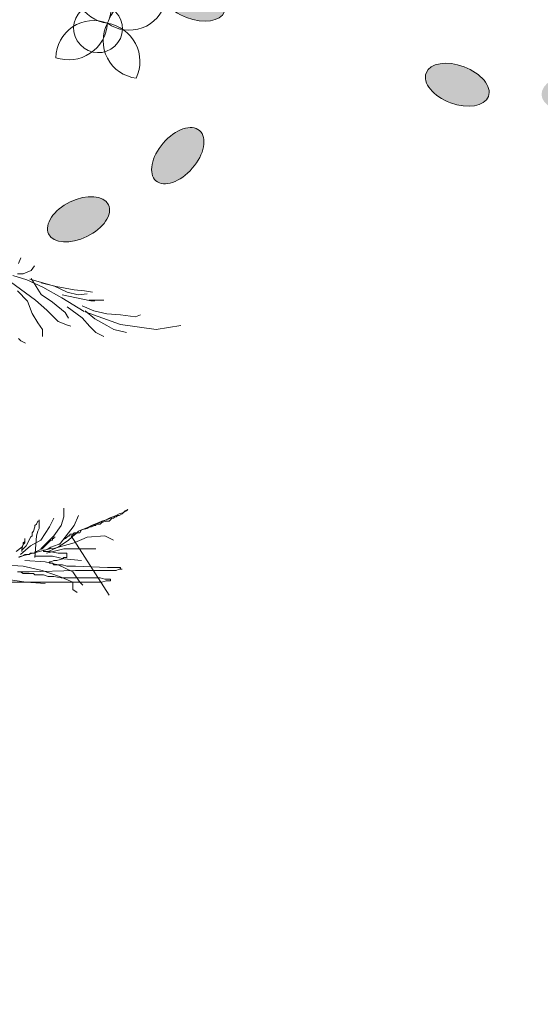
# Model space of a CAD drawing. Units: millimetres. Extents: x 595116 to 630915, y 909473 to 920225.
# Tile 75 of 134: x 629636.47 to 629646.73, y 919266.51 to 919285.9. Entities that reach past the tile are written whole.
import ezdxf

# ---------------------------------------------------------------- set-up
doc = ezdxf.new("R2010")
doc.units = ezdxf.units.MM
doc.layers.add('Dimension', color=3, linetype='Continuous', lineweight=18)
doc.layers.add('L-PLNT', color=85, linetype='Continuous', lineweight=13)
doc.styles.get("Standard").update_dxf_attribs({"font": 'arial.ttf'})
doc.dimstyles.new('ISO-25', dxfattribs={"dimtxt": 9, "dimasz": 6, "dimexe": 1.25, "dimexo": 0.625, "dimtad": 1, "dimlunit": 4, "dimtxsty": 'Standard', "dimcen": 2.5, "dimadec": 0, "dimazin": 0, "dimtfac": 1, "dimtmove": 0, "dimatfit": 3, "dimfxl": 1, "dimarcsym": 0})

# ---------------------------------------------------------------- blocks, each defined once
blk = doc.blocks.new('A$C4FB75ABC')
for p, q in [((4.5963, 3.4774), (4.6082, 3.5072)), ((4.6619, 3.4416), (4.6798, 3.4655)), ((4.5657, 3.4153), (4.6395, 3.3917)), ((4.5903, 3.4238), (4.6201, 3.4238)), ((4.6201, 3.4238), (4.6619, 3.4416)), ((4.5545, 3.382), (4.6858, 3.2866)), ((4.6395, 3.3917), (4.7247, 3.3534)), ((4.6551, 3.396), (4.7847, 3.3597)), ((4.6619, 3.3999), (4.7156, 3.3164)), ((4.7156, 3.3761), (4.7931, 3.3582)), ((4.7847, 3.3597), (4.8521, 3.3286)), ((4.7931, 3.3582), (4.8886, 3.3403)), ((4.5903, 3.3343), (4.644, 3.2807)), ((4.7156, 3.3164), (4.7752, 3.2747)), ((4.7247, 3.3534), (4.8242, 3.2989)), ((4.8262, 3.3131), (4.9765, 3.282)), ((4.8521, 3.3286), (4.9091, 3.3131)), ((4.8886, 3.3403), (4.9422, 3.3343)), ((4.9091, 3.3131), (4.9558, 3.3183)), ((4.9422, 3.3343), (4.984, 3.3284)), ((4.644, 3.2807), (4.6679, 3.2151)), ((4.6858, 3.2866), (4.7454, 3.233)), ((4.7752, 3.2747), (4.8408, 3.2211)), ((4.8242, 3.2989), (4.9411, 3.2265)), ((4.9299, 3.2561), (4.9921, 3.2302)), ((4.9661, 3.2866), (5.0079, 3.2866)), ((4.9765, 3.282), (4.9973, 3.282)), ((5.0079, 3.2866), (5.0437, 3.2866)), ((4.6679, 3.2151), (4.6977, 3.1674)), ((4.7454, 3.233), (4.8051, 3.1734)), ((4.8408, 3.2211), (4.8587, 3.1912)), ((4.8521, 3.2509), (4.9299, 3.1939)), ((4.9454, 3.2302), (4.9973, 3.1887)), ((4.9454, 3.225), (5.1321, 3.1576)), ((4.9921, 3.2302), (5.0595, 3.2146)), ((5.0595, 3.2146), (5.1321, 3.2094)), ((5.1321, 3.2094), (5.2099, 3.1991)), ((5.2099, 3.1991), (5.2358, 3.2094)), ((4.6977, 3.1674), (4.7215, 3.1316)), ((4.8051, 3.1734), (4.8528, 3.1555)), ((4.8528, 3.1555), (4.8707, 3.1495)), ((4.9299, 3.1939), (4.9713, 3.1472)), ((4.9973, 3.1887), (5.0595, 3.1524)), ((5.0595, 3.1524), (5.0958, 3.1317)), ((5.1321, 3.1576), (5.3187, 3.1317)), ((5.3187, 3.1317), (5.4484, 3.1524)), ((4.7215, 3.1316), (4.7215, 3.0959)), ((4.9713, 3.1472), (5.0025, 3.1162)), ((5.0025, 3.1162), (5.0439, 3.0954)), ((5.0958, 3.1317), (5.1632, 3.1162)), ((4.5963, 3.0839), (4.6082, 3.072)), ((4.6082, 3.072), (4.6321, 3.0601)), ((4.835, 2.1495), (4.835, 2.1952)), ((5.1477, 2.1724), (5.1248, 2.1648)), ((5.1401, 2.1648), (5.1477, 2.1724)), ((5.1477, 2.1724), (5.1629, 2.18)), ((5.1553, 2.18), (5.1477, 2.1724)), ((5.1706, 2.1876), (5.1553, 2.18)), ((5.1629, 2.18), (5.1706, 2.1876)), ((4.6901, 2.1114), (4.6977, 2.1266)), ((4.6977, 2.1266), (4.7054, 2.1266)), ((4.7054, 2.1266), (4.7054, 2.1343)), ((4.7054, 2.1343), (4.7054, 2.0885)), ((4.7587, 2.0961), (4.7816, 2.1419)), ((4.8198, 2.1038), (4.835, 2.1495)), ((4.8884, 2.1038), (4.9113, 2.1571)), ((4.9113, 2.0733), (5.079, 2.1419)), ((5.018, 2.119), (4.9799, 2.1038)), ((5.0333, 2.1266), (5.018, 2.119)), ((5.0257, 2.1114), (5.0333, 2.119)), ((5.0562, 2.1343), (5.0333, 2.1266)), ((5.0333, 2.119), (5.0562, 2.1266)), ((5.0714, 2.1419), (5.0562, 2.1343)), ((5.0562, 2.1266), (5.0714, 2.1266)), ((5.1095, 2.1571), (5.0714, 2.1419)), ((5.0714, 2.1266), (5.079, 2.1343)), ((5.079, 2.1343), (5.0867, 2.1419)), ((5.0867, 2.1419), (5.0943, 2.1419)), ((5.0943, 2.1419), (5.1019, 2.1495)), ((5.1019, 2.1495), (5.1095, 2.1495)), ((5.1248, 2.1648), (5.1095, 2.1571)), ((5.1095, 2.1495), (5.1172, 2.1571)), ((5.1172, 2.1571), (5.1248, 2.1571)), ((5.1248, 2.1571), (5.1401, 2.1648)), ((4.6672, 2.0657), (4.6749, 2.0733)), ((4.6749, 2.0733), (4.6825, 2.0961)), ((4.6825, 2.1038), (4.6901, 2.1114)), ((4.6825, 2.0961), (4.6825, 2.1038)), ((4.6977, 2.0733), (4.6901, 2.0504)), ((4.7054, 2.0885), (4.6977, 2.0733)), ((4.713, 2.0275), (4.7587, 2.0961)), ((4.7816, 2.0504), (4.8198, 2.1038)), ((4.8121, 2.0047), (4.8884, 2.1038)), ((4.8579, 2.0275), (4.9113, 2.0733)), ((4.9036, 2.0657), (4.9113, 2.0733)), ((4.9113, 2.0733), (4.9265, 2.0809)), ((4.9265, 2.0809), (4.9189, 2.0657)), ((4.9265, 2.0809), (4.957, 2.0885)), ((4.9494, 2.0885), (4.9265, 2.0809)), ((4.9799, 2.1038), (4.9494, 2.0885)), ((4.957, 2.0885), (4.9723, 2.0961)), ((4.9723, 2.0961), (4.9799, 2.0961)), ((4.9799, 2.0961), (4.9952, 2.1038)), ((4.9952, 2.1038), (5.0028, 2.1038)), ((5.0028, 2.1038), (5.0028, 2.1114)), ((5.0028, 2.1114), (5.0257, 2.1114)), ((4.6215, 2.0123), (4.6291, 2.0199)), ((4.6291, 2.0199), (4.6291, 2.0352)), ((4.6291, 2.0352), (4.6291, 2.0123)), ((4.6444, 2.0123), (4.6596, 2.0428)), ((4.6596, 2.0428), (4.6672, 2.0504)), ((4.6596, 1.9971), (4.713, 2.0275)), ((4.6672, 2.0504), (4.6672, 2.0657)), ((4.6901, 2.0504), (4.6825, 1.9361)), ((4.713, 1.9818), (4.7816, 2.0504)), ((4.7664, 2.0275), (4.7511, 2.0123)), ((4.774, 2.0275), (4.7664, 2.0275)), ((4.7816, 2.0352), (4.774, 2.0352)), ((4.774, 2.0352), (4.774, 2.0275)), ((4.7892, 2.0428), (4.7816, 2.0428)), ((4.7816, 2.0428), (4.7816, 2.0352)), ((4.8045, 1.9894), (4.8579, 2.0275)), ((4.8198, 2.0123), (4.8274, 2.0275)), ((4.8274, 2.0275), (4.8426, 2.0352)), ((4.8426, 2.0352), (4.8579, 2.0504)), ((4.8579, 2.0504), (4.8655, 2.0504)), ((4.8655, 2.0504), (4.8655, 2.058)), ((4.8655, 2.058), (4.8808, 2.058)), ((4.8808, 2.0504), (4.8731, 2.0504)), ((4.8731, 2.0504), (5.0714, 1.7379)), ((4.8808, 2.058), (4.8884, 2.0657)), ((4.896, 2.058), (4.8808, 2.058)), ((4.8808, 2.058), (4.8808, 2.0504)), ((4.8884, 2.0657), (4.9036, 2.0657)), ((4.8884, 2.0123), (4.957, 2.0428)), ((4.9036, 2.0657), (4.896, 2.058)), ((4.9189, 2.0657), (4.9036, 2.0657)), ((4.957, 2.0428), (5.0485, 2.0504)), ((5.0485, 2.0504), (5.0943, 2.0275)), ((4.5833, 1.9666), (4.6138, 1.9894)), ((4.7725, 1.9851), (4.5975, 1.9398)), ((4.6062, 1.9513), (4.6596, 1.9971)), ((4.6138, 1.9894), (4.6215, 2.0047)), ((4.6215, 2.0047), (4.6138, 1.9818)), ((4.6138, 1.9818), (4.6138, 1.9666)), ((4.6138, 1.9742), (4.6215, 1.9818)), ((4.6138, 1.9666), (4.6138, 1.9742)), ((4.6215, 2.0047), (4.6215, 2.0123)), ((4.6291, 2.0123), (4.6215, 2.0047)), ((4.6215, 1.9818), (4.6367, 1.9971)), ((4.6367, 1.9971), (4.6444, 2.0123)), ((4.6901, 1.9666), (4.6825, 1.9589)), ((4.7054, 1.9742), (4.6901, 1.9666)), ((4.7206, 1.9818), (4.7054, 1.9742)), ((4.7359, 1.9971), (4.7206, 1.9818)), ((4.7282, 1.9666), (4.7282, 1.9742)), ((4.7282, 1.9742), (4.7359, 1.9742)), ((4.7587, 1.9666), (4.7282, 1.9666)), ((4.7435, 2.0047), (4.7359, 1.9971)), ((4.7359, 1.9742), (4.7511, 1.9818)), ((4.7511, 2.0123), (4.7435, 2.0047)), ((4.7435, 1.9589), (4.835, 1.9818)), ((4.7511, 1.9818), (4.7664, 1.9894)), ((4.7511, 1.9666), (4.8045, 1.9894)), ((4.8045, 1.9589), (4.7587, 1.9666)), ((4.7664, 1.9894), (4.8045, 2.0047)), ((4.774, 1.9818), (4.8884, 2.0123)), ((4.8045, 2.0047), (4.8198, 2.0123)), ((4.835, 1.9818), (4.9494, 1.9818)), ((4.9494, 1.9818), (5.0028, 1.9818)), ((4.6138, 1.9437), (4.5986, 1.9361)), ((4.6291, 1.9513), (4.6138, 1.9437)), ((4.652, 1.9513), (4.6291, 1.9513)), ((4.6291, 1.9208), (4.7359, 1.9132)), ((4.6596, 1.9589), (4.652, 1.9513)), ((4.6825, 1.9589), (4.6596, 1.9589)), ((4.6825, 1.9437), (4.774, 1.9437)), ((4.7359, 1.9132), (4.8045, 1.898)), ((4.7587, 1.9056), (4.7587, 1.9132)), ((4.7587, 1.9132), (4.7664, 1.9132)), ((4.7664, 1.9132), (4.7816, 1.9208)), ((4.774, 1.9437), (4.835, 1.9285)), ((4.7816, 1.9208), (4.7969, 1.9208)), ((4.7969, 1.9208), (4.8274, 1.9285)), ((4.8503, 1.9589), (4.8045, 1.9589)), ((4.8274, 1.9285), (4.835, 1.9361)), ((4.835, 1.9361), (4.8503, 1.9361)), ((4.835, 1.9285), (4.9265, 1.9208)), ((4.8503, 1.9361), (4.8503, 1.9589)), ((4.5071, 1.898), (4.6215, 1.8903)), ((4.6062, 1.8599), (4.591, 1.8599)), ((4.591, 1.8599), (4.652, 1.8599)), ((4.6215, 1.8522), (4.6062, 1.8599)), ((4.6215, 1.8903), (4.7206, 1.8675)), ((4.652, 1.8599), (4.896, 1.8675)), ((4.7206, 1.8675), (4.8121, 1.837)), ((4.774, 1.9056), (4.7587, 1.9056)), ((4.7816, 1.898), (4.774, 1.9056)), ((4.8274, 1.898), (4.7816, 1.898)), ((4.8045, 1.898), (4.8808, 1.8599)), ((4.8503, 1.8903), (4.8274, 1.898)), ((4.896, 1.8903), (4.8503, 1.8903)), ((4.8808, 1.8599), (4.9189, 1.8065)), ((5.0638, 1.8827), (4.896, 1.8903)), ((4.896, 1.8675), (5.1095, 1.8675)), ((5.1324, 1.8827), (5.0638, 1.8827)), ((5.1095, 1.8675), (5.1248, 1.8751)), ((5.1248, 1.8751), (5.1401, 1.8751)), ((5.1324, 1.8751), (5.1324, 1.8827)), ((5.1401, 1.8751), (5.1324, 1.8751)), ((4.53, 1.8217), (4.6367, 1.8065)), ((4.6749, 1.8522), (4.6215, 1.8522)), ((4.6825, 1.8446), (4.6749, 1.8522)), ((4.7282, 1.8446), (4.6825, 1.8446)), ((4.7511, 1.837), (4.7282, 1.8446)), ((4.7816, 1.837), (4.7511, 1.837)), ((4.8198, 1.8294), (4.7816, 1.837)), ((4.8121, 1.837), (4.8808, 1.8065)), ((5.0257, 1.8294), (4.8198, 1.8294)), ((5.0485, 1.8217), (5.0257, 1.8294)), ((5.0333, 1.8065), (5.0562, 1.8141)), ((5.079, 1.8217), (5.0485, 1.8217)), ((5.0562, 1.8141), (5.079, 1.8141)), ((5.079, 1.8141), (5.079, 1.8217)), ((4.1639, 1.8065), (5.0333, 1.8065)), ((4.6367, 1.8065), (4.7359, 1.7989)), ((4.8808, 1.8065), (4.8808, 1.7684)), ((4.8808, 1.7684), (4.9036, 1.7531)), ((4.9189, 1.8065), (4.9341, 1.7913))]:
    blk.add_line(p, q)
blk = doc.blocks.new('A$C77972600')
h = blk.add_hatch(color=256)
edge = h.paths.add_edge_path()
edge.add_ellipse((3.2403, 1.6985), major_axis=(-0.1668, -0.0838), ratio=0.578492, start_angle=0, end_angle=360, ccw=False)
edge = h.paths.add_edge_path()
edge.add_ellipse((4.2796, 1.6084), major_axis=(-0.1206, -0.1425), ratio=0.578492, start_angle=0, end_angle=360, ccw=False)
edge = h.paths.add_edge_path()
edge.add_ellipse((4.7739, 0.881), major_axis=(-0.1747, 0.0657), ratio=0.578492, start_angle=0, end_angle=360, ccw=False)
edge = h.paths.add_edge_path()
edge.add_ellipse((5.4333, 0.8328), major_axis=(-0.1865, -0.008), ratio=0.578492, start_angle=0, end_angle=360, ccw=False)
edge = h.paths.add_edge_path()
edge.add_ellipse((4.6573, 4.2045), major_axis=(-0.1865, -0.008), ratio=0.578492, start_angle=0, end_angle=360, ccw=False)
edge = h.paths.add_edge_path()
edge.add_ellipse((4.556, 3.4032), major_axis=(-0.1865, -0.008), ratio=0.578492, start_angle=0, end_angle=360, ccw=False)
edge = h.paths.add_edge_path()
edge.add_ellipse((4.9297, 3.677), major_axis=(-0.1668, -0.0838), ratio=0.578492, start_angle=0, end_angle=360, ccw=False)
edge = h.paths.add_edge_path()
edge.add_ellipse((3.7756, 2.5742), major_axis=(-0.1206, -0.1425), ratio=0.578492, start_angle=0, end_angle=360, ccw=False)
edge = h.paths.add_edge_path()
edge.add_ellipse((3.1788, 2.8466), major_axis=(-0.1206, -0.1425), ratio=0.578492, start_angle=0, end_angle=360, ccw=False)
edge = h.paths.add_edge_path()
edge.add_ellipse((3.8763, 3.0252), major_axis=(-0.1206, -0.1425), ratio=0.578492, start_angle=0, end_angle=360, ccw=False)
edge = h.paths.add_edge_path()
edge.add_ellipse((2.3609, 1.8217), major_axis=(-0.1865, -0.008), ratio=0.578492, start_angle=0, end_angle=360, ccw=False)
edge = h.paths.add_edge_path()
edge.add_ellipse((3.0627, 1.8578), major_axis=(-0.1865, -0.008), ratio=0.578492, start_angle=0, end_angle=360, ccw=False)
edge = h.paths.add_edge_path()
edge.add_ellipse((2.7605, 2.0535), major_axis=(-0.1865, -0.008), ratio=0.578492, start_angle=0, end_angle=360, ccw=False)
edge = h.paths.add_edge_path()
edge.add_ellipse((2.1439, 3.4246), major_axis=(-0.1668, -0.0838), ratio=0.578492, start_angle=0, end_angle=360, ccw=False)
edge = h.paths.add_edge_path()
edge.add_ellipse((4.2959, 2.0225), major_axis=(-0.1747, 0.0657), ratio=0.578492, start_angle=0, end_angle=360, ccw=False)
edge = h.paths.add_edge_path()
edge.add_ellipse((1.9127, 4.2528), major_axis=(-0.1865, -0.008), ratio=0.578492, start_angle=0, end_angle=360, ccw=False)
edge = h.paths.add_edge_path()
edge.add_ellipse((1.5555, 4.1052), major_axis=(-0.1747, 0.0657), ratio=0.578492, start_angle=0, end_angle=360, ccw=False)
edge = h.paths.add_edge_path()
edge.add_ellipse((0.9962, 4.2695), major_axis=(-0.1865, -0.008), ratio=0.578492, start_angle=0, end_angle=360, ccw=False)
edge = h.paths.add_edge_path()
edge.add_ellipse((1.2179, 3.5926), major_axis=(-0.1747, 0.0657), ratio=0.578492, start_angle=0, end_angle=360, ccw=False)
edge = h.paths.add_edge_path()
edge.add_ellipse((1.6764, 3.6493), major_axis=(-0.1747, 0.0657), ratio=0.578492, start_angle=0, end_angle=360, ccw=False)
edge = h.paths.add_edge_path()
edge.add_ellipse((0.8384, 2.8599), major_axis=(-0.1668, -0.0838), ratio=0.578492, start_angle=0, end_angle=360, ccw=False)
edge = h.paths.add_edge_path()
edge.add_ellipse((0.9659, 2.049), major_axis=(-0.1206, -0.1425), ratio=0.578492, start_angle=0, end_angle=360, ccw=False)
edge = h.paths.add_edge_path()
edge.add_ellipse((1.3147, 2.1383), major_axis=(-0.1206, -0.1425), ratio=0.578492, start_angle=0, end_angle=360, ccw=False)
edge = h.paths.add_edge_path()
edge.add_ellipse((5.4586, 2.9929), major_axis=(-0.1865, -0.008), ratio=0.578492, start_angle=0, end_angle=360, ccw=False)
edge = h.paths.add_edge_path()
edge.add_ellipse((3.4224, 5.3915), major_axis=(-0.1865, -0.008), ratio=0.578492, start_angle=0, end_angle=360, ccw=False)
edge = h.paths.add_edge_path()
edge.add_ellipse((3.7245, 5.1958), major_axis=(-0.1865, -0.008), ratio=0.578492, start_angle=0, end_angle=360, ccw=False)
edge = h.paths.add_edge_path()
edge.add_ellipse((4.5588, 5.4431), major_axis=(-0.1668, -0.0838), ratio=0.578492, start_angle=0, end_angle=360, ccw=False)
edge = h.paths.add_edge_path()
edge.add_ellipse((4.4393, 4.7252), major_axis=(-0.1668, -0.0838), ratio=0.578492, start_angle=0, end_angle=360, ccw=False)
edge = h.paths.add_edge_path()
edge.add_ellipse((4.7087, 5.1006), major_axis=(-0.1668, -0.0838), ratio=0.578492, start_angle=0, end_angle=360, ccw=False)
edge = h.paths.add_edge_path()
edge.add_ellipse((3.7138, 4.6852), major_axis=(-0.1668, -0.0838), ratio=0.578492, start_angle=0, end_angle=360, ccw=False)
h = blk.add_hatch(color=256)
edge = h.paths.add_edge_path()
edge.add_ellipse((4.1652, 1.933), major_axis=(0.1866, 0.0058), ratio=0.578492, start_angle=0, end_angle=360)
edge = h.paths.add_edge_path()
edge.add_ellipse((3.2944, 1.3586), major_axis=(0.1739, -0.0678), ratio=0.578492, start_angle=0, end_angle=360)
edge = h.paths.add_edge_path()
edge.add_ellipse((3.2064, 0.4835), major_axis=(0.1223, 0.141), ratio=0.578492, start_angle=0, end_angle=360)
edge = h.paths.add_edge_path()
edge.add_ellipse((2.6497, 0.127), major_axis=(0.1678, 0.0818), ratio=0.578492, start_angle=0, end_angle=360)
edge = h.paths.add_edge_path()
edge.add_ellipse((1.7252, 3.461), major_axis=(0.1678, 0.0818), ratio=0.578492, start_angle=0, end_angle=360)
edge = h.paths.add_edge_path()
edge.add_ellipse((2.1962, 2.8048), major_axis=(0.1678, 0.0818), ratio=0.578492, start_angle=0, end_angle=360)
edge = h.paths.add_edge_path()
edge.add_ellipse((1.7372, 2.8674), major_axis=(0.1866, 0.0058), ratio=0.578492, start_angle=0, end_angle=360)
edge = h.paths.add_edge_path()
edge.add_ellipse((3.2773, 2.4479), major_axis=(0.1739, -0.0678), ratio=0.578492, start_angle=0, end_angle=360)
edge = h.paths.add_edge_path()
edge.add_ellipse((3.6722, 2.9717), major_axis=(0.1739, -0.0678), ratio=0.578492, start_angle=0, end_angle=360)
edge = h.paths.add_edge_path()
edge.add_ellipse((2.9739, 2.7963), major_axis=(0.1739, -0.0678), ratio=0.578492, start_angle=0, end_angle=360)
edge = h.paths.add_edge_path()
edge.add_ellipse((4.8796, 2.4604), major_axis=(0.1678, 0.0818), ratio=0.578492, start_angle=0, end_angle=360)
edge = h.paths.add_edge_path()
edge.add_ellipse((4.2454, 2.1577), major_axis=(0.1678, 0.0818), ratio=0.578492, start_angle=0, end_angle=360)
edge = h.paths.add_edge_path()
edge.add_ellipse((4.4178, 2.4738), major_axis=(0.1678, 0.0818), ratio=0.578492, start_angle=0, end_angle=360)
edge = h.paths.add_edge_path()
edge.add_ellipse((4.3066, 3.973), major_axis=(0.1866, 0.0058), ratio=0.578492, start_angle=0, end_angle=360)
edge = h.paths.add_edge_path()
edge.add_ellipse((3.0828, 1.7149), major_axis=(0.1223, 0.141), ratio=0.578492, start_angle=0, end_angle=360)
edge = h.paths.add_edge_path()
edge.add_ellipse((4.1152, 4.8113), major_axis=(0.1678, 0.0818), ratio=0.578492, start_angle=0, end_angle=360)
edge = h.paths.add_edge_path()
edge.add_ellipse((4.4995, 4.8518), major_axis=(0.1223, 0.141), ratio=0.578492, start_angle=0, end_angle=360)
edge = h.paths.add_edge_path()
edge.add_ellipse((4.913, 5.2627), major_axis=(0.1678, 0.0818), ratio=0.578492, start_angle=0, end_angle=360)
edge = h.paths.add_edge_path()
edge.add_ellipse((5.0407, 4.562), major_axis=(0.1223, 0.141), ratio=0.578492, start_angle=0, end_angle=360)
edge = h.paths.add_edge_path()
edge.add_ellipse((4.6105, 4.3933), major_axis=(0.1223, 0.141), ratio=0.578492, start_angle=0, end_angle=360)
edge = h.paths.add_edge_path()
edge.add_ellipse((5.7235, 4.0986), major_axis=(0.1866, 0.0058), ratio=0.578492, start_angle=0, end_angle=360)
edge = h.paths.add_edge_path()
edge.add_ellipse((5.9977, 3.3249), major_axis=(0.1739, -0.0678), ratio=0.578492, start_angle=0, end_angle=360)
edge = h.paths.add_edge_path()
edge.add_ellipse((5.6486, 3.2372), major_axis=(0.1739, -0.0678), ratio=0.578492, start_angle=0, end_angle=360)
edge = h.paths.add_edge_path()
edge.add_ellipse((1.5981, 2.014), major_axis=(0.1678, 0.0818), ratio=0.578492, start_angle=0, end_angle=360)
edge = h.paths.add_edge_path()
edge.add_ellipse((2.2453, 5.0931), major_axis=(0.1678, 0.0818), ratio=0.578492, start_angle=0, end_angle=360)
edge = h.paths.add_edge_path()
edge.add_ellipse((2.073, 4.777), major_axis=(0.1678, 0.0818), ratio=0.578492, start_angle=0, end_angle=360)
edge = h.paths.add_edge_path()
edge.add_ellipse((1.2216, 4.5968), major_axis=(0.1866, 0.0058), ratio=0.578492, start_angle=0, end_angle=360)
edge = h.paths.add_edge_path()
edge.add_ellipse((1.6688, 4.0227), major_axis=(0.1866, 0.0058), ratio=0.578492, start_angle=0, end_angle=360)
edge = h.paths.add_edge_path()
edge.add_ellipse((1.253, 4.2244), major_axis=(0.1866, 0.0058), ratio=0.578492, start_angle=0, end_angle=360)
edge = h.paths.add_edge_path()
edge.add_ellipse((2.3257, 4.3332), major_axis=(0.1866, 0.0058), ratio=0.578492, start_angle=0, end_angle=360)
for centre, radius, start, end in [((2.8419, 1.442), 0.2185, 156.8071, 262.1441), ((2.6229, 1.3182), 0.2106, 333.8874, 85.0638), ((3.0209, 1.1614), 0.2185, 57.5868, 162.9238), ((2.9338, 1.3974), 0.2106, 234.6671, 345.8435), ((2.7336, 1.03), 0.2106, 68.147, 179.3234), ((2.5939, 1.2392), 0.2185, 251.0667, 356.4037), ((2.9982, 1.1271), 0.2106, 152.1384, 263.3149), ((2.7756, 1.0101), 0.2185, 335.0581, 80.3951)]:
    blk.add_arc(centre, radius, start, end)
for centre, major_axis, start_param, end_param in [((3.2944, 1.3586), (-0.1739, 0.0678), 3.141593, 9.424778), ((3.2064, 0.4835), (-0.1223, -0.141), 3.141593, 9.424778), ((2.6497, 0.127), (-0.1678, -0.0818), -1.570796, 4.712389)]:
    blk.add_ellipse(centre, major_axis=major_axis, ratio=0.578492, start_param=start_param, end_param=end_param)
blk.add_ellipse((2.7589, 1.1975), major_axis=(-0.0941, 0.1005), ratio=0.985729)
at = {"extrusion": (0, 0, -1)}
blk.add_ellipse((4.7739, 0.881), major_axis=(-0.1747, 0.0657), ratio=0.578492, dxfattribs=at)
blk = doc.blocks.new('*D211')
at = {"layer": 'Defpoints', "color": 0, "transparency": 16777216}
for p in [(629535.386, 919258.662), (629586.227, 919258.662), (629586.227, 919250.943)]:
    blk.add_point(p, dxfattribs=at)
at = {"layer": 'Dimension', "color": 0, "lineweight": -2, "transparency": 16777216}
for p, q in [((629535.386, 919258.037), (629535.386, 919249.693)), ((629586.227, 919258.037), (629586.227, 919249.693)), ((629541.386, 919250.943), (629580.227, 919250.943)), ((629586.227, 919250.943), (629648.699, 919250.943))]:
    blk.add_line(p, q, dxfattribs=at)
at = {"layer": 'Dimension', "color": 0, "transparency": 16777216}
for points in [[(629541.386, 919251.943), (629541.386, 919249.943), (629535.386, 919250.943)], [(629580.227, 919251.943), (629580.227, 919249.943), (629586.227, 919250.943)]]:
    blk.add_solid(points, dxfattribs=at)
at = {"layer": 'Dimension', "color": 0, "transparency": 16777216, "insert": (629620.463, 919256.167), "char_height": 9, "attachment_point": 5}
blk.add_mtext('4\'-3" TYP.', dxfattribs=at)
blk = doc.blocks.new('*D216')
at = {"layer": 'Defpoints', "color": 0, "transparency": 16777216}
for p in [(629743.541, 919411.928), (629505.041, 919411.828), (629743.541, 918832.378)]:
    blk.add_point(p, dxfattribs=at)
at = {"layer": 'Dimension', "color": 0, "lineweight": -2, "transparency": 16777216}
for p, q in [((629505.041, 919411.203), (629505.041, 918831.128)), ((629743.541, 919411.303), (629743.541, 918831.128)), ((629511.041, 918832.378), (629737.541, 918832.378))]:
    blk.add_line(p, q, dxfattribs=at)
at = {"layer": 'Dimension', "color": 0, "transparency": 16777216}
for points in [[(629511.041, 918833.378), (629511.041, 918831.378), (629505.041, 918832.378)], [(629737.541, 918833.378), (629737.541, 918831.378), (629743.541, 918832.378)]]:
    blk.add_solid(points, dxfattribs=at)
at = {"layer": 'Dimension', "color": 0, "transparency": 16777216, "insert": (629624.291, 918837.656), "char_height": 9, "attachment_point": 5}
blk.add_mtext('19\'-10 1/2"', dxfattribs=at)

msp = doc.modelspace()

# ---------------------------------------------------------------- block references
at = {"layer": 'L-PLNT'}
for name, p, xscale, yscale, zscale in [('A$C77972600', (629628.32, 919281.523), 3.512546757812034, 3.512546757812034, 3.512546757812034), ('A$C4FB75ABC', (629619.193, 919268.043), 3.753413438031968, 3.753413438031968, 3.753413438031968)]:
    msp.add_blockref(name, p, dxfattribs=dict(at, xscale=xscale, yscale=yscale, zscale=zscale))

# ---------------------------------------------------------------- dimensions: what is measured, and where the dimension line sits
at = {"layer": 'Dimension'}
dim = msp.add_linear_dim(base=(629743.541, 918832.378), p1=(629505.041, 919411.828), p2=(629743.541, 919411.928), dimstyle='ISO-25', override={"dimdec": 1, "dimlfac": 1, "dimrnd": 0, "dimzin": 1, "dimdsep": 46, "dimlunit": 4, "dimfrac": 2}, dxfattribs=at)
dim.commit()
dim.dimension.update_dxf_attribs({"geometry": '*D216', "text_midpoint": (629624.291, 918837.656)})
dim = msp.add_linear_dim(base=(629586.227, 919250.943), p1=(629535.386, 919258.662), p2=(629586.227, 919258.662), text='<> TYP.', dimstyle='ISO-25', override={"dimdec": 1, "dimlfac": 1, "dimrnd": 0, "dimzin": 1, "dimdsep": 46, "dimlunit": 4, "dimfrac": 2}, dxfattribs=at)
dim.commit()
dim.dimension.update_dxf_attribs({"geometry": '*D211', "text_midpoint": (629620.463, 919256.167)})

doc.saveas('drawing.dxf')
